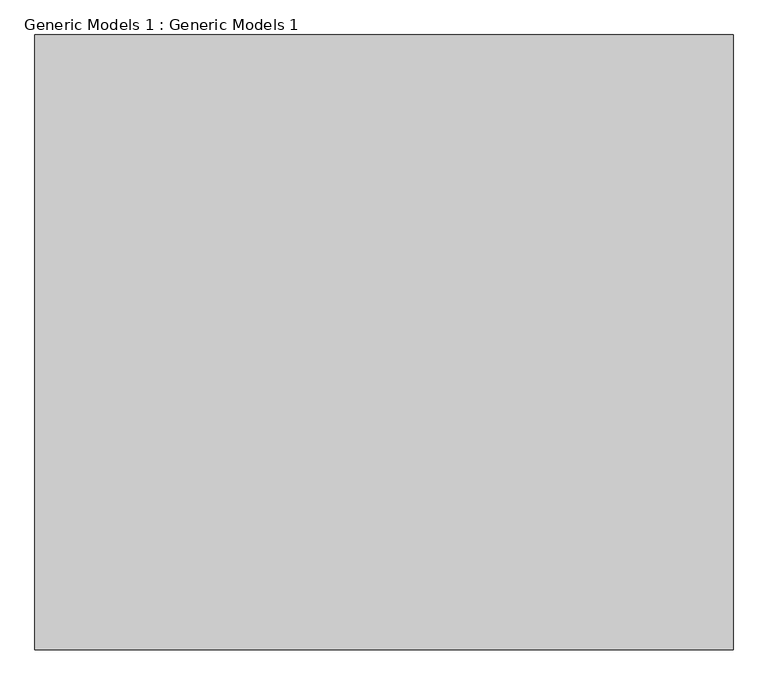
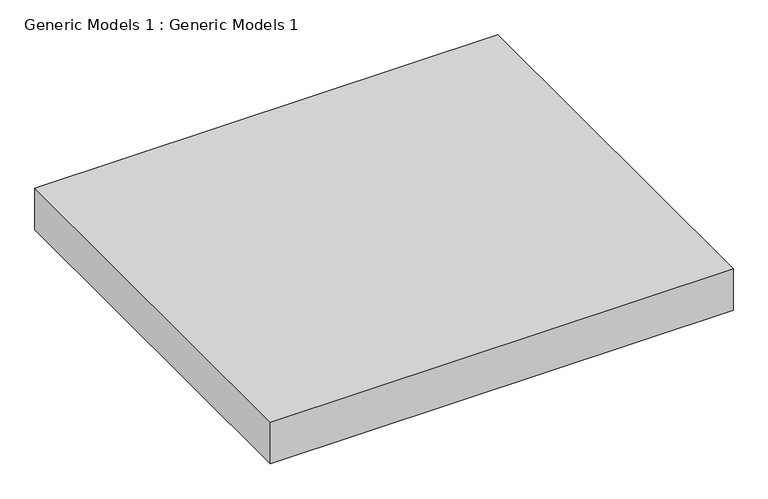
"""IFC4 building model written with IfcOpenShell, lengths in millimetres: proxy geometry, Generic Models 1 : Generic Models 1."""

from ifc_helpers import new_model, si_unit, origin, origin_with_axes, place, context, project, spatial, polyline, outline, extrude, source, transform, mapped, element, save


def generic_models_1_generic_models_1_34925b1c(model_context):
    return source(origin(), model_context, "Body", "SweptSolid", [
        extrude(outline(polyline([(-5897.9859258, -8981.6777232), (-5897.9859258, -11801.0777232), (-9098.3859258, -11801.0777232), (-9098.3859258, -8981.6777232), (-5897.9859258, -8981.6777232)])), origin_with_axes(), (0.0, 0.0, 1.0), 304.8),
    ])


if __name__ == "__main__":
    model = new_model("IFC4")
    model_context = context("Model", 3, world=origin())
    ifc_project = project(units=[si_unit("LENGTHUNIT", "METRE", prefix="MILLI")], contexts=[model_context])
    site = spatial("IfcSite", under=ifc_project)
    building = spatial("IfcBuilding", under=site)
    placement = place(None, origin())
    generic_models_1_generic_models_1_shape = generic_models_1_generic_models_1_34925b1c(model_context)
    element("IfcBuildingElementProxy", 1, Name="Generic Models 1 : Generic Models 1", ObjectType="Generic Models 1 : Generic Models 1", at=placement, inside=building, context=model_context, shape_type="MappedRepresentation", body=[
        mapped(generic_models_1_generic_models_1_shape, transform((0.0, 0.0, 0.0), x_axis=(1.0, 0.0, 0.0), y_axis=(0.0, 1.0, 0.0), z_axis=(0.0, 0.0, 1.0))),
    ])
    save(model, "model.ifc")
